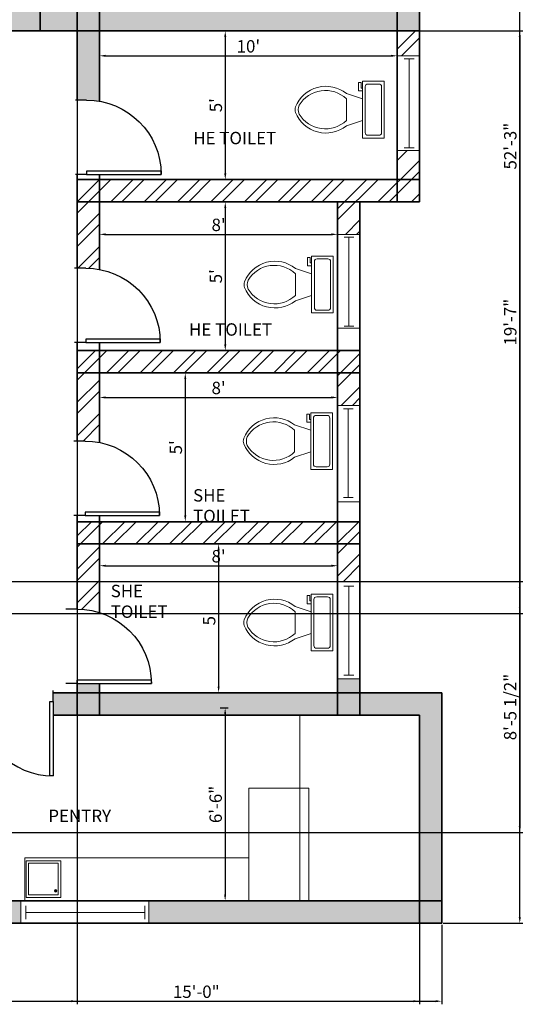
# Model space of a CAD drawing. Units: millimetres. Extents: x 2436 to 3005, y 774 to 1472.
# Tile 2 of 3: x 2799 to 3005, y 774 to 1172. Entities that reach past the tile are written whole.
import ezdxf

# ---------------------------------------------------------------- set-up
doc = ezdxf.new("R2010")
doc.units = ezdxf.units.MM
for name, color, linetype, lineweight in [('A-ANNO-DIMS', 2, 'Continuous', 18), ('A-AREA-IDEN', 10, 'Continuous', 25), ('A-FLOR-CASE', 140, 'Continuous', 18), ('A-FLOR-FIXT', 140, 'Continuous', 18), ('A-WALL-PATT', 3, 'Continuous', 13), ('doors', 30, 'Continuous', 25), ('walls', 80, 'Continuous', 35), ('window', 190, 'Continuous', 20)]:
    doc.layers.add(name, color=color, linetype=linetype, lineweight=lineweight)
doc.styles.get("Standard").update_dxf_attribs({"font": 'arial.ttf'})
doc.dimstyles.new('ISO-25', dxfattribs={"dimtxt": 5, "dimasz": 2.5, "dimexe": 1.25, "dimexo": 0.625, "dimtad": 1, "dimdec": 0, "dimlunit": 3, "dimtxsty": 'Standard', "dimcen": 2.5, "dimadec": 0, "dimazin": 0, "dimtfac": 1, "dimtdec": 0, "dimtmove": 0, "dimatfit": 3, "dimfxl": 1, "dimarcsym": 0})

# ---------------------------------------------------------------- blocks, each defined once
blk = doc.blocks.new('*U2')
for p, q in [((0, 0), (0, -6)), ((40, 0), (40, -6))]:
    blk.add_line(p, q)
blk.add_lwpolyline([(0, 0), (0, 40), (1.75, 40), (1.75, 0)], close=True)
blk.add_arc((0, 0), 40, 0, 90)
blk = doc.blocks.new('*U4')
for p, q in [((0, 4), (0, 0)), ((36, 4), (36, 0)), ((0, 2), (36, 2))]:
    blk.add_line(p, q)
blk = doc.blocks.new('*U5')
for p, q in [((0, 4), (0, 0)), ((36, 4), (36, 0)), ((0, 2), (36, 2))]:
    blk.add_line(p, q)
blk = doc.blocks.new('Toilet - top')
for p, q in [((9.5, -6), (9.5, -2)), ((-10, -8.5), (-8, -8.5)), ((-10, -9.5), (-10, -8.5)), ((-7, -9.5), (-10, -9.5)), ((-8, -8.5), (-8, -8)), ((-7, -8), (-7, -9.5)), ((-4, -8), (-6, -14)), ((4, -8), (6, -14)), ((4, -14), (-4, -14))]:
    blk.add_line(p, q)
blk.add_lwpolyline([(10.5, -8), (10.5, 0), (-10.5, 0), (-10.5, -8)], close=True)
for points in [[(-9.5, -2), (-9.5, -6)], [(8.5, -1), (-8.5, -1)], [(-8.5, -7), (8.5, -7)]]:
    blk.add_lwpolyline(points)
for centre, radius, start, end in [((-8.62, -1.88), 0.884, 81.8699, 188.1301), ((8.62, -1.88), 0.884, 351.8699, 98.1301), ((-8.62, -6.12), 0.884, 171.8699, 278.1301), ((8.62, -6.12), 0.884, 261.8699, 8.1301), ((3.52, -21.58), 12.17, 141.4691, 247.9714), ((4.2, -21.82), 11.33, 136.3677, 238.9468), ((-3.52, -21.58), 12.17, 292.0284, 38.5307), ((-4.2, -21.82), 11.33, 301.053, 43.6321), ((0, -27.88), 4, 245.7318, 294.2682), ((0, -29), 4, 254.8605, 285.1395)]:
    blk.add_arc(centre, radius, start, end)
blk = doc.blocks.new('*D25')
at = {"layer": 'A-ANNO-DIMS', "color": 0, "lineweight": -2, "transparency": 16777216}
for p, q in [((2879.98, 893.97), (2883.19, 893.97)), ((2881.94, 891.47), (2881.94, 818.62)), ((2879.98, 816.12), (2883.19, 816.12))]:
    blk.add_line(p, q, dxfattribs=at)
at = {"layer": 'A-ANNO-DIMS', "color": 0, "transparency": 16777216}
for points in [[(2881.52, 891.47), (2882.35, 891.47), (2881.94, 893.97)], [(2881.52, 818.62), (2882.35, 818.62), (2881.94, 816.12)]]:
    blk.add_solid(points, dxfattribs=at)
at = {"layer": 'Defpoints', "color": 0, "transparency": 16777216}
for p in [(2879.35, 893.97), (2879.35, 816.12), (2881.94, 816.12)]:
    blk.add_point(p, dxfattribs=at)
at = {"layer": 'A-ANNO-DIMS', "color": 0, "transparency": 16777216, "insert": (2878.76, 855.05), "char_height": 5, "attachment_point": 5, "rotation": 90}
blk.add_mtext('6\'-6"', dxfattribs=at)
blk = doc.blocks.new('*D26')
at = {"layer": 'A-ANNO-DIMS', "color": 0, "lineweight": -2, "transparency": 16777216}
for p, q in [((2879.3, 957.62), (2879.3, 902.62)), ((2879.92, 960.12), (2880.55, 960.12)), ((2879.92, 900.12), (2880.55, 900.12))]:
    blk.add_line(p, q, dxfattribs=at)
at = {"layer": 'A-ANNO-DIMS', "color": 0, "transparency": 16777216}
for points in [[(2878.88, 957.62), (2879.72, 957.62), (2879.3, 960.12)], [(2878.88, 902.62), (2879.72, 902.62), (2879.3, 900.12)]]:
    blk.add_solid(points, dxfattribs=at)
at = {"layer": 'Defpoints', "color": 0, "transparency": 16777216}
for p in [(2879.3, 960.12), (2879.3, 900.12), (2879.3, 900.12)]:
    blk.add_point(p, dxfattribs=at)
at = {"layer": 'A-ANNO-DIMS', "color": 0, "transparency": 16777216, "insert": (2876.13, 930.12), "char_height": 5, "attachment_point": 5, "rotation": 90}
blk.add_mtext("5'", dxfattribs=at)
blk = doc.blocks.new('*D27')
at = {"layer": 'A-ANNO-DIMS', "color": 0, "lineweight": -2, "transparency": 16777216}
for p, q in [((2831.3, 1019.85), (2831.3, 1020.48)), ((2833.8, 1019.23), (2924.8, 1019.23)), ((2927.3, 1019.85), (2927.3, 1020.48))]:
    blk.add_line(p, q, dxfattribs=at)
at = {"layer": 'A-ANNO-DIMS', "color": 0, "transparency": 16777216}
for points in [[(2833.8, 1019.65), (2833.8, 1018.81), (2831.3, 1019.23)], [(2924.8, 1019.65), (2924.8, 1018.81), (2927.3, 1019.23)]]:
    blk.add_solid(points, dxfattribs=at)
at = {"layer": 'Defpoints', "color": 0, "transparency": 16777216}
for p in [(2831.3, 1019.23), (2927.3, 1019.23), (2927.3, 1019.23)]:
    blk.add_point(p, dxfattribs=at)
at = {"layer": 'A-ANNO-DIMS', "color": 0, "transparency": 16777216, "insert": (2879.3, 1022.41), "char_height": 5, "attachment_point": 5}
blk.add_mtext("8'", dxfattribs=at)
blk = doc.blocks.new('*D28')
at = {"layer": 'A-ANNO-DIMS', "color": 0, "lineweight": -2, "transparency": 16777216}
for p, q in [((2881.99, 1164.62), (2881.99, 1109.62)), ((2882.61, 1167.12), (2883.24, 1167.12)), ((2882.61, 1107.12), (2883.24, 1107.12))]:
    blk.add_line(p, q, dxfattribs=at)
at = {"layer": 'A-ANNO-DIMS', "color": 0, "transparency": 16777216}
for points in [[(2881.57, 1164.62), (2882.4, 1164.62), (2881.99, 1167.12)], [(2881.57, 1109.62), (2882.4, 1109.62), (2881.99, 1107.12)]]:
    blk.add_solid(points, dxfattribs=at)
at = {"layer": 'Defpoints', "color": 0, "transparency": 16777216}
for p in [(2881.99, 1167.12), (2881.99, 1107.12), (2881.99, 1107.12)]:
    blk.add_point(p, dxfattribs=at)
at = {"layer": 'A-ANNO-DIMS', "color": 0, "transparency": 16777216, "insert": (2878.82, 1137.12), "char_height": 5, "attachment_point": 5, "rotation": 90}
blk.add_mtext("5'", dxfattribs=at)
blk = doc.blocks.new('*D29')
at = {"layer": 'A-ANNO-DIMS', "color": 0, "lineweight": -2, "transparency": 16777216}
for p, q in [((2882.61, 1098.12), (2883.24, 1098.12)), ((2881.99, 1095.62), (2881.99, 1040.62)), ((2882.61, 1038.12), (2883.24, 1038.12))]:
    blk.add_line(p, q, dxfattribs=at)
at = {"layer": 'A-ANNO-DIMS', "color": 0, "transparency": 16777216}
for points in [[(2881.57, 1095.62), (2882.4, 1095.62), (2881.99, 1098.12)], [(2881.57, 1040.62), (2882.4, 1040.62), (2881.99, 1038.12)]]:
    blk.add_solid(points, dxfattribs=at)
at = {"layer": 'Defpoints', "color": 0, "transparency": 16777216}
for p in [(2881.99, 1098.12), (2881.99, 1038.12), (2881.99, 1038.12)]:
    blk.add_point(p, dxfattribs=at)
at = {"layer": 'A-ANNO-DIMS', "color": 0, "transparency": 16777216, "insert": (2878.82, 1068.12), "char_height": 5, "attachment_point": 5, "rotation": 90}
blk.add_mtext("5'", dxfattribs=at)
blk = doc.blocks.new('*D30')
at = {"layer": 'A-ANNO-DIMS', "color": 0, "lineweight": -2, "transparency": 16777216}
for p, q in [((2866.48, 1029.12), (2867.11, 1029.12)), ((2865.86, 1026.62), (2865.86, 971.62)), ((2866.48, 969.12), (2867.11, 969.12))]:
    blk.add_line(p, q, dxfattribs=at)
at = {"layer": 'A-ANNO-DIMS', "color": 0, "transparency": 16777216}
for points in [[(2865.44, 1026.62), (2866.28, 1026.62), (2865.86, 1029.12)], [(2865.44, 971.62), (2866.28, 971.62), (2865.86, 969.12)]]:
    blk.add_solid(points, dxfattribs=at)
at = {"layer": 'Defpoints', "color": 0, "transparency": 16777216}
for p in [(2865.86, 1029.12), (2865.86, 969.12), (2865.86, 969.12)]:
    blk.add_point(p, dxfattribs=at)
at = {"layer": 'A-ANNO-DIMS', "color": 0, "transparency": 16777216, "insert": (2862.69, 999.12), "char_height": 5, "attachment_point": 5, "rotation": 90}
blk.add_mtext("5'", dxfattribs=at)
blk = doc.blocks.new('*D31')
at = {"layer": 'A-ANNO-DIMS', "color": 0, "lineweight": -2, "transparency": 16777216}
for p, q in [((2831.3, 951.41), (2831.3, 950.1)), ((2833.8, 951.35), (2924.8, 951.35)), ((2927.3, 951.98), (2927.3, 952.6))]:
    blk.add_line(p, q, dxfattribs=at)
at = {"layer": 'A-ANNO-DIMS', "color": 0, "transparency": 16777216}
for points in [[(2833.8, 951.77), (2833.8, 950.93), (2831.3, 951.35)], [(2924.8, 951.77), (2924.8, 950.93), (2927.3, 951.35)]]:
    blk.add_solid(points, dxfattribs=at)
at = {"layer": 'Defpoints', "color": 0, "transparency": 16777216}
for p in [(2831.3, 952.04), (2927.3, 951.35), (2927.3, 951.35)]:
    blk.add_point(p, dxfattribs=at)
at = {"layer": 'A-ANNO-DIMS', "color": 0, "transparency": 16777216, "insert": (2879.3, 954.53), "char_height": 5, "attachment_point": 5}
blk.add_mtext("8'", dxfattribs=at)
blk = doc.blocks.new('*D32')
at = {"layer": 'A-ANNO-DIMS', "color": 0, "lineweight": -2, "transparency": 16777216}
for p, q in [((2831.3, 1156.81), (2831.3, 1155.81)), ((2833.8, 1157.06), (2948.8, 1157.06)), ((2951.3, 1156.81), (2951.3, 1155.81))]:
    blk.add_line(p, q, dxfattribs=at)
at = {"layer": 'A-ANNO-DIMS', "color": 0, "transparency": 16777216}
for points in [[(2833.8, 1157.47), (2833.8, 1156.64), (2831.3, 1157.06)], [(2948.8, 1157.47), (2948.8, 1156.64), (2951.3, 1157.06)]]:
    blk.add_solid(points, dxfattribs=at)
at = {"layer": 'Defpoints', "color": 0, "transparency": 16777216}
for p in [(2831.3, 1157.43), (2951.3, 1157.43), (2951.3, 1157.06)]:
    blk.add_point(p, dxfattribs=at)
at = {"layer": 'A-ANNO-DIMS', "color": 0, "transparency": 16777216, "insert": (2891.3, 1160.23), "char_height": 5, "attachment_point": 5}
blk.add_mtext("10'", dxfattribs=at)
blk = doc.blocks.new('*D33')
at = {"layer": 'A-ANNO-DIMS', "color": 0, "lineweight": -2, "transparency": 16777216}
for p, q in [((2831.3, 1087.23), (2831.3, 1083.77)), ((2833.8, 1085.02), (2924.8, 1085.02)), ((2927.3, 1085.65), (2927.3, 1086.27))]:
    blk.add_line(p, q, dxfattribs=at)
at = {"layer": 'A-ANNO-DIMS', "color": 0, "transparency": 16777216}
for points in [[(2833.8, 1085.44), (2833.8, 1084.61), (2831.3, 1085.02)], [(2924.8, 1085.44), (2924.8, 1084.61), (2927.3, 1085.02)]]:
    blk.add_solid(points, dxfattribs=at)
at = {"layer": 'Defpoints', "color": 0, "transparency": 16777216}
for p in [(2831.3, 1087.86), (2927.3, 1085.02), (2927.3, 1085.02)]:
    blk.add_point(p, dxfattribs=at)
at = {"layer": 'A-ANNO-DIMS', "color": 0, "transparency": 16777216, "insert": (2879.3, 1088.2), "char_height": 5, "attachment_point": 5}
blk.add_mtext("8'", dxfattribs=at)
blk = doc.blocks.new('*D40')
at = {"layer": 'A-ANNO-DIMS', "color": 0, "lineweight": -2, "transparency": 16777216}
for p, q in [((2480.3, 806.5), (2480.3, 774.42)), ((2969.3, 806.5), (2969.3, 774.42)), ((2482.8, 775.67), (2966.8, 775.67))]:
    blk.add_line(p, q, dxfattribs=at)
at = {"layer": 'A-ANNO-DIMS', "color": 0, "transparency": 16777216}
for points in [[(2482.8, 776.09), (2482.8, 775.26), (2480.3, 775.67)], [(2966.8, 776.09), (2966.8, 775.26), (2969.3, 775.67)]]:
    blk.add_solid(points, dxfattribs=at)
at = {"layer": 'Defpoints', "color": 0, "transparency": 16777216}
for p in [(2480.3, 807.12), (2969.3, 807.12), (2969.3, 775.67)]:
    blk.add_point(p, dxfattribs=at)
at = {"layer": 'A-ANNO-DIMS', "color": 0, "transparency": 16777216, "insert": (2724.8, 778.85), "char_height": 5, "attachment_point": 5}
blk.add_mtext('40\'-9"', dxfattribs=at)
blk = doc.blocks.new('*D41')
at = {"layer": 'A-ANNO-DIMS', "color": 0, "lineweight": -2, "transparency": 16777216}
for p, q in [((2960.92, 1434.12), (3002, 1434.12)), ((3000.75, 809.62), (3000.75, 1431.62)), ((2969.92, 807.12), (3002, 807.12))]:
    blk.add_line(p, q, dxfattribs=at)
at = {"layer": 'A-ANNO-DIMS', "color": 0, "transparency": 16777216}
for points in [[(3000.33, 1431.62), (3001.17, 1431.62), (3000.75, 1434.12)], [(3000.33, 809.62), (3001.17, 809.62), (3000.75, 807.12)]]:
    blk.add_solid(points, dxfattribs=at)
at = {"layer": 'Defpoints', "color": 0, "transparency": 16777216}
for p in [(2960.3, 1434.12), (3000.75, 1434.12), (2969.3, 807.12)]:
    blk.add_point(p, dxfattribs=at)
at = {"layer": 'A-ANNO-DIMS', "color": 0, "transparency": 16777216, "insert": (2997.57, 1120.62), "char_height": 5, "attachment_point": 5, "rotation": 90}
blk.add_mtext('52\'-3"', dxfattribs=at)
blk = doc.blocks.new('*D42')
at = {"layer": 'A-ANNO-DIMS', "color": 0, "lineweight": -2, "transparency": 16777216}
for p, q in [((2780.3, 931.5), (2780.3, 774.42)), ((2960.3, 890.5), (2960.3, 774.42)), ((2782.8, 775.67), (2957.8, 775.67))]:
    blk.add_line(p, q, dxfattribs=at)
at = {"layer": 'A-ANNO-DIMS', "color": 0, "transparency": 16777216}
for points in [[(2782.8, 776.09), (2782.8, 775.26), (2780.3, 775.67)], [(2957.8, 776.09), (2957.8, 775.26), (2960.3, 775.67)]]:
    blk.add_solid(points, dxfattribs=at)
at = {"layer": 'Defpoints', "color": 0, "transparency": 16777216}
for p in [(2780.3, 932.12), (2960.3, 891.12), (2960.3, 775.67)]:
    blk.add_point(p, dxfattribs=at)
at = {"layer": 'A-ANNO-DIMS', "color": 0, "transparency": 16777216, "insert": (2870.3, 778.85), "char_height": 5, "attachment_point": 5}
blk.add_mtext('15\'-0"', dxfattribs=at)
blk = doc.blocks.new('*D43')
at = {"layer": 'A-ANNO-DIMS', "color": 0, "lineweight": -2, "transparency": 16777216}
for p, q in [((2822.3, 1175.5), (2822.3, 774.42)), ((2618.3, 1160.31), (2618.3, 774.42)), ((2620.8, 775.67), (2819.8, 775.67))]:
    blk.add_line(p, q, dxfattribs=at)
at = {"layer": 'A-ANNO-DIMS', "color": 0, "transparency": 16777216}
for points in [[(2620.8, 776.09), (2620.8, 775.26), (2618.3, 775.67)], [(2819.8, 776.09), (2819.8, 775.26), (2822.3, 775.67)]]:
    blk.add_solid(points, dxfattribs=at)
at = {"layer": 'Defpoints', "color": 0, "transparency": 16777216}
for p in [(2822.3, 1176.12), (2618.3, 1160.93), (2822.3, 775.67)]:
    blk.add_point(p, dxfattribs=at)
at = {"layer": 'A-ANNO-DIMS', "color": 0, "transparency": 16777216, "insert": (2720.3, 778.85), "char_height": 5, "attachment_point": 5}
blk.add_mtext('17\'-0"', dxfattribs=at)
blk = doc.blocks.new('*D44')
at = {"layer": 'A-ANNO-DIMS', "color": 0, "lineweight": -2, "transparency": 16777216}
for p, q in [((2798.92, 1167.12), (3002, 1167.12)), ((3000.75, 1164.62), (3000.75, 934.62)), ((2780.92, 932.12), (3002, 932.12))]:
    blk.add_line(p, q, dxfattribs=at)
at = {"layer": 'A-ANNO-DIMS', "color": 0, "transparency": 16777216}
for points in [[(3000.33, 1164.62), (3001.17, 1164.62), (3000.75, 1167.12)], [(3000.33, 934.62), (3001.17, 934.62), (3000.75, 932.12)]]:
    blk.add_solid(points, dxfattribs=at)
at = {"layer": 'Defpoints', "color": 0, "transparency": 16777216}
for p in [(2798.3, 1167.12), (2780.3, 932.12), (3000.75, 932.12)]:
    blk.add_point(p, dxfattribs=at)
at = {"layer": 'A-ANNO-DIMS', "color": 0, "transparency": 16777216, "insert": (2997.57, 1049.62), "char_height": 5, "attachment_point": 5, "rotation": 90}
blk.add_mtext('19\'-7"', dxfattribs=at)
blk = doc.blocks.new('*D54')
at = {"layer": 'A-ANNO-DIMS', "color": 0, "lineweight": -2, "transparency": 16777216}
for p, q in [((2543.78, 945.02), (3002, 945.02)), ((3000.75, 942.52), (3000.75, 846.17)), ((2543.78, 843.67), (3002, 843.67))]:
    blk.add_line(p, q, dxfattribs=at)
at = {"layer": 'A-ANNO-DIMS', "color": 0, "transparency": 16777216}
for points in [[(3000.33, 942.52), (3001.17, 942.52), (3000.75, 945.02)], [(3000.33, 846.17), (3001.17, 846.17), (3000.75, 843.67)]]:
    blk.add_solid(points, dxfattribs=at)
at = {"layer": 'Defpoints', "color": 0, "transparency": 16777216}
for p in [(2543.16, 945.02), (2543.16, 843.67), (3000.75, 843.67)]:
    blk.add_point(p, dxfattribs=at)
at = {"layer": 'A-ANNO-DIMS', "color": 0, "transparency": 16777216, "insert": (2997.54, 894.35), "char_height": 5, "attachment_point": 5, "rotation": 90}
blk.add_mtext('8\'-5 1/2"', dxfattribs=at)

msp = doc.modelspace()

# ---------------------------------------------------------------- hatches: boundary and pattern name
at = {"layer": 'A-WALL-PATT'}
h = msp.add_hatch(color=256, dxfattribs=at)
h.dxf.hatch_style = 1
h.paths.add_polyline_path([(2822.3, 1374.12), (2489.3, 1374.12), (2489.3, 1365.12), (2822.3, 1365.12)])
h.paths.add_polyline_path([(2831.3, 1374.12), (2822.3, 1374.12), (2822.3, 1365.12), (2831.3, 1365.12)])
h.paths.add_polyline_path([(2831.3, 1365.12), (2822.3, 1365.12), (2822.3, 1353.75), (2824.37, 1353.75, -0.041466), (2831.3, 1353.17)])
h.paths.add_polyline_path([(2960.3, 1425.12), (2951.3, 1425.12), (2951.3, 1305.12), (2960.3, 1305.12)])
h.paths.add_polyline_path([(2960.3, 1434.12), (2951.3, 1434.12), (2951.3, 1425.12), (2960.3, 1425.12)])
h.paths.add_polyline_path([(2951.3, 1434.12), (2831.3, 1434.12), (2831.3, 1425.12), (2951.3, 1425.12)])
h.paths.add_polyline_path([(2831.3, 1434.12), (2822.3, 1434.12), (2822.3, 1425.12), (2831.3, 1425.12)])
h.paths.add_polyline_path([(2489.3, 1374.12), (2480.3, 1374.12), (2480.3, 1365.12), (2489.3, 1365.12)])
h.paths.add_polyline_path([(2489.3, 1365.12), (2480.3, 1365.12), (2480.3, 1354.49), (2489.3, 1354.89)])
h.paths.add_polyline_path([(2489.3, 1313.48, -0.04329), (2482.1, 1312.53), (2480.3, 1312.44), (2480.3, 1176.12), (2489.3, 1176.12)])
h.paths.add_polyline_path([(2489.3, 1176.12), (2480.3, 1176.12), (2480.3, 1167.12), (2489.3, 1167.12)])
h.paths.add_polyline_path([(2609.3, 1176.12), (2489.3, 1176.12), (2489.3, 1167.12), (2609.3, 1167.12)])
h.paths.add_polyline_path([(2625.3, 1176.12), (2618.3, 1176.12), (2618.3, 1167.12), (2625.3, 1167.12)])
h.paths.add_polyline_path([(2618.3, 1176.12), (2616.3, 1176.12), (2616.3, 1167.12), (2618.3, 1167.12)])
h.paths.add_polyline_path([(2616.3, 1176.12), (2609.3, 1176.12), (2609.3, 1167.12), (2616.3, 1167.12)])
h.paths.add_polyline_path([(2618.3, 1167.12), (2609.3, 1167.12), (2609.3, 1160.63, -0.029892), (2614.31, 1160.93), (2618.3, 1160.93)])
h.paths.add_polyline_path([(2625.3, 1305.12), (2616.3, 1305.12), (2616.3, 1176.12), (2618.3, 1176.12), (2625.3, 1176.12)])
h.paths.add_polyline_path([(2798.3, 1176.12), (2625.3, 1176.12), (2625.3, 1167.12), (2798.3, 1167.12)])
h.paths.add_polyline_path([(2807.3, 1176.12), (2798.3, 1176.12), (2798.3, 1167.12), (2807.3, 1167.12)])
h.paths.add_polyline_path([(2831.3, 1176.12), (2822.3, 1176.12), (2822.3, 1167.12), (2831.3, 1167.12)])
h.paths.add_polyline_path([(2822.3, 1176.12), (2807.3, 1176.12), (2807.3, 1167.12), (2822.3, 1167.12)])
h.paths.add_polyline_path([(2951.3, 1176.12), (2831.3, 1176.12), (2831.3, 1167.12), (2951.3, 1167.12)])
h.paths.add_polyline_path([(2960.3, 1176.12), (2951.3, 1176.12), (2951.3, 1167.12), (2960.3, 1167.12)])
h.paths.add_polyline_path([(2960.3, 1296.12), (2951.3, 1296.12), (2951.3, 1176.12), (2960.3, 1176.12)])
h.paths.add_polyline_path([(2960.3, 1305.12), (2951.3, 1305.12), (2951.3, 1296.12), (2960.3, 1296.12)])
h.paths.add_polyline_path([(2951.3, 1305.12), (2831.3, 1305.12), (2831.3, 1296.12), (2951.3, 1296.12)])
h.paths.add_polyline_path([(2822.3, 1305.12), (2807.3, 1305.12), (2807.3, 1296.12), (2822.3, 1296.12)])
h.paths.add_polyline_path([(2831.3, 1305.12), (2822.3, 1305.12), (2822.3, 1296.12), (2831.3, 1296.12)])
h.paths.add_polyline_path([(2831.3, 1311.75), (2824.37, 1311.75), (2822.3, 1311.75), (2822.3, 1305.12), (2831.3, 1305.12)])
h.paths.add_polyline_path([(2807.3, 1305.12), (2798.3, 1305.12), (2798.3, 1296.12), (2807.3, 1296.12)])
h.paths.add_polyline_path([(2807.3, 1236.01), (2798.3, 1236.01), (2798.3, 1221.93), (2801.81, 1221.93, -0.032777), (2807.3, 1221.57)])
h.paths.add_polyline_path([(2831.3, 1167.12), (2822.3, 1167.12), (2822.3, 1139.2), (2826.09, 1139.2, -0.043681), (2831.3, 1138.75)])
h.paths.add_polyline_path([(2807.3, 1179.93), (2801.81, 1179.93), (2798.3, 1179.93), (2798.3, 1176.12), (2807.3, 1176.12)])
h.paths.add_polyline_path([(2927.3, 900.12), (2831.3, 900.12), (2831.3, 891.12), (2927.3, 891.12)])
h.paths.add_polyline_path([(2936.3, 900.12), (2927.3, 900.12), (2927.3, 891.12), (2936.3, 891.12)])
h.paths.add_polyline_path([(2936.3, 905.69), (2927.3, 905.69), (2927.3, 900.12), (2936.3, 900.12)])
h.paths.add_polyline_path([(2831.3, 900.12), (2822.3, 900.12), (2822.3, 891.12), (2831.3, 891.12)])
h.paths.add_polyline_path([(2831.3, 903.84), (2822.3, 903.84), (2822.3, 900.12), (2831.3, 900.12)])
h.paths.add_polyline_path([(2822.3, 900.12), (2812.6, 900.12), (2812.6, 896.54), (2812.6, 891.12), (2822.3, 891.12)])
h.paths.add_polyline_path([(2969.3, 900.12), (2958.95, 900.12), (2936.3, 900.12), (2936.3, 891.12), (2960.3, 891.12), (2960.3, 826.87), (2960.3, 816.12), (2969.3, 816.12), (2969.3, 826.87), (2969.3, 891.12)])
h = msp.add_hatch(color=256, dxfattribs=at)
h.dxf.hatch_style = 1
h.paths.add_polyline_path([(2780.3, 891.12), (2771.3, 891.12), (2771.3, 816.12), (2780.3, 816.12)])
h.paths.add_polyline_path([(2780.3, 900.12), (2771.3, 900.12), (2771.3, 891.12), (2780.3, 891.12)])
h.paths.add_polyline_path([(2780.3, 923.12), (2771.3, 923.12), (2771.3, 900.12), (2780.3, 900.12)])
h.paths.add_polyline_path([(2780.3, 932.12), (2771.3, 932.12), (2771.3, 923.12), (2780.3, 923.12)])
h.paths.add_polyline_path([(2771.3, 932.12), (2687.55, 932.12), (2687.55, 930.04), (2687.55, 923.12), (2771.3, 923.12)])
h.paths.add_polyline_path([(2651.3, 923.12), (2642.3, 923.12), (2642.3, 816.12), (2651.3, 816.12)])
h.paths.add_polyline_path([(2651.3, 816.12), (2642.3, 816.12), (2642.3, 807.12), (2651.3, 807.12)])
h.paths.add_polyline_path([(2771.3, 816.12), (2651.3, 816.12), (2651.3, 807.12), (2771.3, 807.12)])
h.paths.add_polyline_path([(2780.3, 816.12), (2771.3, 816.12), (2771.3, 807.12), (2780.3, 807.12)])
h.paths.add_polyline_path([(2799.5, 816.12), (2780.3, 816.12), (2780.3, 807.12), (2799.5, 807.12)])
h.paths.add_polyline_path([(2960.3, 816.12), (2851.13, 816.12), (2851.13, 807.12), (2960.3, 807.12)])
h.paths.add_polyline_path([(2969.3, 816.12), (2960.3, 816.12), (2960.3, 807.12), (2969.3, 807.12)])
h.paths.add_polyline_path([(2642.3, 816.12), (2489.3, 816.12), (2489.3, 807.12), (2642.3, 807.12)])
h.paths.add_polyline_path([(2489.3, 816.12), (2480.3, 816.12), (2480.3, 807.12), (2489.3, 807.12)])
h.paths.add_polyline_path([(2489.3, 969.12), (2480.3, 969.12), (2480.3, 816.12), (2489.3, 816.12)])
h.paths.add_polyline_path([(2609.3, 978.12), (2489.3, 978.12), (2489.3, 969.12), (2609.3, 969.12)])
h.paths.add_polyline_path([(2489.3, 978.12), (2480.3, 978.12), (2480.3, 969.12), (2489.3, 969.12)])
h.paths.add_polyline_path([(2618.3, 978.12), (2609.3, 978.12), (2609.3, 969.12), (2618.3, 969.12)])
h.paths.add_polyline_path([(2642.3, 978.12), (2618.3, 978.12), (2618.3, 969.12), (2642.3, 969.12)])
h.paths.add_polyline_path([(2651.3, 978.12), (2642.3, 978.12), (2642.3, 969.12), (2651.3, 969.12)])
h.paths.add_polyline_path([(2651.3, 969.12), (2642.3, 969.12), (2642.3, 964.63), (2651.3, 964.63)])
h.paths.add_polyline_path([(2651.3, 932.12), (2642.3, 932.12), (2642.3, 923.12), (2651.3, 923.12)])
h.paths.add_polyline_path([(2657.55, 930.04), (2657.55, 932.12), (2651.3, 932.12), (2651.3, 923.12), (2658.36, 923.12, -0.058212)])
h.paths.add_polyline_path([(2651.3, 938.64, -0.080735), (2642.3, 935.23), (2642.3, 932.12), (2651.3, 932.12)])
h.paths.add_polyline_path([(2489.3, 1038.12), (2480.3, 1038.12), (2480.3, 978.12), (2489.3, 978.12)])
h.paths.add_polyline_path([(2618.3, 987.5), (2609.3, 987.5), (2609.3, 978.12), (2618.3, 978.12)])
h.paths.add_polyline_path([(2618.3, 1038.12), (2609.3, 1038.12), (2609.3, 1026.42), (2618.3, 1026.42)])
h.paths.add_polyline_path([(2489.3, 1047.12), (2480.3, 1047.12), (2480.3, 1038.12), (2489.3, 1038.12)])
h.paths.add_polyline_path([(2618.3, 1047.12), (2609.3, 1047.12), (2609.3, 1038.12), (2618.3, 1038.12)])
h.paths.add_polyline_path([(2489.3, 1167.12), (2480.3, 1167.12), (2480.3, 1047.12), (2489.3, 1047.12)])
h.paths.add_polyline_path([(2618.3, 1118.93), (2614.31, 1118.93), (2609.3, 1118.93), (2609.3, 1108.92), (2618.3, 1108.92)])
h.paths.add_polyline_path([(2618.3, 1056.71), (2609.3, 1056.71), (2609.3, 1047.12), (2618.3, 1047.12)])
edge = h.paths.add_edge_path()
edge.add_arc((2601.4, 1049.98), 30, 185.4674, 203.2834)
edge.add_line((2573.84, 1038.12), (2489.3, 1038.12))
edge.add_line((2489.3, 1038.12), (2489.3, 1047.12))
edge.add_line((2489.3, 1047.12), (2571.54, 1047.12))
h.paths.add_polyline_path([(2601.4, 1047.12), (2601.4, 1038.12), (2609.3, 1038.12), (2609.3, 1047.12)])
h = msp.add_hatch(dxfattribs=at)
h.set_pattern_fill('ANSI32', color=256)
h.paths.add_polyline_path([(2951.3, 1107.12), (2831.3, 1107.12), (2831.3, 1098.12), (2951.3, 1098.12)])
h.paths.add_polyline_path([(2831.3, 1107.12), (2822.3, 1107.12), (2822.3, 1098.12), (2831.3, 1098.12)])
h.paths.add_polyline_path([(2831.3, 1098.12), (2822.3, 1098.12), (2822.3, 1071.38), (2825.75, 1071.38, -0.046499), (2831.3, 1070.86)])
h.paths.add_polyline_path([(2936.3, 1098.12), (2927.3, 1098.12), (2927.3, 1085.02), (2936.3, 1085.02)])
h.paths.add_polyline_path([(2960.3, 1107.12), (2951.3, 1107.12), (2951.3, 1098.12), (2960.3, 1098.12)])
h.paths.add_polyline_path([(2960.3, 1118.92), (2951.3, 1118.92), (2951.3, 1107.12), (2960.3, 1107.12)])
h.paths.add_polyline_path([(2960.3, 1167.12), (2951.3, 1167.12), (2951.3, 1157.06), (2960.3, 1157.06)])
h.paths.add_polyline_path([(2927.3, 1037.38), (2927.3, 1038.12), (2831.3, 1038.12), (2831.3, 1037.38), (2831.3, 1029.12), (2927.3, 1029.12)])
h.paths.add_polyline_path([(2936.3, 1037.38), (2936.3, 1038.12), (2927.3, 1038.12), (2927.3, 1037.38), (2927.3, 1029.12), (2936.3, 1029.12)])
h.paths.add_polyline_path([(2831.3, 1029.12), (2822.3, 1029.12), (2822.3, 1001.65), (2825.44, 1001.65, -0.049211), (2831.3, 1001.07)])
h.paths.add_polyline_path([(2831.3, 1037.38), (2831.3, 1038.12), (2822.3, 1038.12), (2822.3, 1029.12), (2831.3, 1029.12)])
h.paths.add_polyline_path([(2927.3, 969.12), (2831.3, 969.12), (2831.3, 960.12), (2927.3, 960.12)])
h.paths.add_polyline_path([(2831.3, 969.12), (2822.3, 969.12), (2822.3, 960.12), (2831.3, 960.12)])
h.paths.add_polyline_path([(2831.3, 960.12), (2822.3, 960.12), (2822.3, 933.84, -0.076367), (2831.3, 932.43)])
h.paths.add_polyline_path([(2936.3, 969.12), (2927.3, 969.12), (2927.3, 960.12), (2936.3, 960.12)])
h.paths.add_polyline_path([(2936.3, 960.12), (2927.3, 960.12), (2927.3, 945.01), (2936.3, 945.01), (2936.3, 949.23)])
h.paths.add_polyline_path([(2936.3, 1029.12), (2927.3, 1029.12), (2927.3, 1015.96), (2936.3, 1015.96)])

# ---------------------------------------------------------------- linework, layer by layer
at = {"layer": 'A-FLOR-CASE'}
for p, q in [((2912.09, 816.12), (2912.09, 891.12)), ((2891.47, 833.51), (2801.13, 833.51)), ((2801.13, 833.51), (2801.13, 816.12)), ((2801.13, 816.12), (2912.09, 816.12))]:
    msp.add_line(p, q, dxfattribs=at)
msp.add_lwpolyline([(2891.47, 816.12), (2915.69, 816.12), (2915.69, 861.56), (2891.47, 861.56)], close=True, dxfattribs=at)
at = {"layer": 'A-FLOR-FIXT'}
for points in [[(2801.67, 832.31), (2815.64, 832.31), (2815.64, 817.57), (2801.67, 817.57)], [(2802.67, 831.31), (2814.64, 831.31), (2814.64, 818.57), (2802.67, 818.57)]]:
    msp.add_lwpolyline(points, close=True, dxfattribs=at)
for radius in [0.499, 0.13]:
    msp.add_circle((2813.59, 820.2), radius, dxfattribs=at)
at = {"layer": 'walls'}
for p, q in [((2951.3, 1434.12), (2951.3, 1098.12)), ((2960.3, 1434.12), (2960.3, 1098.12)), ((2807.3, 1181.77), (2807.3, 1167.12)), ((2822.3, 1176.12), (2822.3, 1139.2)), ((2831.3, 1176.12), (2831.3, 1138.75)), ((2960.3, 1167.12), (2480.3, 1167.12)), ((2822.3, 1109.2), (2822.3, 1098.12)), ((2831.3, 1109.2), (2831.3, 1098.12)), ((2960.3, 1107.12), (2822.3, 1107.12)), ((2960.3, 1098.12), (2822.3, 1098.12)), ((2822.3, 1098.12), (2822.3, 1071.38)), ((2831.3, 1098.12), (2831.3, 1070.86)), ((2927.3, 1098.12), (2927.3, 1037.38)), ((2960.3, 1098.12), (2936.3, 1098.12)), ((2960.3, 1098.12), (2936.3, 1098.12)), ((2936.3, 1098.12), (2936.3, 1037.38)), ((2822.3, 1041.38), (2822.3, 1001.65)), ((2831.3, 1041.38), (2831.3, 1037.38)), ((2936.3, 1038.12), (2822.3, 1038.12)), ((2831.3, 1037.38), (2831.3, 1001.07)), ((2927.3, 1037.38), (2927.3, 981.58)), ((2936.3, 1037.38), (2936.3, 981.58)), ((2936.3, 1029.12), (2822.3, 1029.12)), ((2927.3, 981.58), (2927.3, 951.35)), ((2936.3, 981.58), (2936.3, 949.23)), ((2822.3, 971.65), (2822.3, 960.12)), ((2831.3, 971.65), (2831.3, 932.43)), ((2936.3, 969.12), (2822.3, 969.12)), ((2936.3, 960.12), (2822.3, 960.12)), ((2822.3, 960.12), (2822.3, 933.84)), ((2927.3, 960.12), (2927.3, 891.12)), ((2936.3, 949.23), (2936.3, 891.12)), ((2822.3, 903.84), (2822.3, 891.12)), ((2831.3, 903.84), (2831.3, 891.12)), ((2936.3, 900.12), (2812.6, 900.12)), ((2936.3, 900.12), (2960.3, 900.12)), ((2969.3, 900.12), (2958.95, 900.12)), ((2969.3, 891.12), (2969.3, 900.12)), ((2936.3, 891.12), (2812.6, 891.12)), ((2936.3, 891.12), (2960.3, 891.12)), ((2960.3, 891.12), (2960.3, 826.87)), ((2969.3, 891.12), (2969.3, 826.87)), ((2960.3, 826.87), (2960.3, 807.12)), ((2969.3, 826.87), (2969.3, 816.12)), ((2969.3, 816.12), (2480.3, 816.12)), ((2969.3, 816.12), (2969.3, 807.12)), ((2969.3, 807.12), (2480.3, 807.12))]:
    msp.add_line(p, q, dxfattribs=at)
at = {"layer": 'window'}
for p, q in [((2951.3, 1157.06), (2960.3, 1157.06)), ((2951.3, 1118.92), (2960.3, 1118.92)), ((2936.3, 1085.02), (2927.3, 1085.02)), ((2927.3, 1047.22), (2936.3, 1047.22)), ((2936.3, 1015.96), (2927.3, 1015.96)), ((2936.3, 977.15), (2927.3, 977.15)), ((2936.3, 945.01), (2927.3, 945.01)), ((2936.3, 905.69), (2927.3, 905.69)), ((2799.5, 816.12), (2799.5, 807.12)), ((2851.13, 816.12), (2851.13, 807.12))]:
    msp.add_line(p, q, dxfattribs=at)

# ---------------------------------------------------------------- block references
at = {"layer": 'A-FLOR-FIXT', "xscale": 1.089104113419681, "yscale": 1.089104113419681, "zscale": 1.089104113419681, "rotation": 270}
for p in [(2946.08, 1135.33), (2925.53, 1064.76), (2925.21, 1001.62), (2925.38, 928.42)]:
    msp.add_blockref('Toilet - top', p, dxfattribs=at)
at = {"layer": 'doors', "yscale": 0.75, "zscale": 0.75}
for p, xscale, rotation in [((2826.09, 1109.2), -0.75, 270), ((2825.75, 1041.38), -0.75, 270), ((2825.44, 971.65), -0.75, 270), ((2822.19, 903.84), -0.75, 270), ((2812.6, 896.54), 0.75, 180)]:
    msp.add_blockref('*U2', p, dxfattribs=dict(at, xscale=xscale, rotation=rotation))
at = {"layer": 'window'}
for name, p, xscale, yscale, zscale, rotation in [('*U5', (2958.11, 1119.95), 0.9968650679331311, 0.9968650679331311, 0.9968650679331311, 90), ('*U5', (2933.87, 1048.05), 0.9968650679331311, 0.9968650679331311, 0.9968650679331311, 90), ('*U5', (2933.6, 978.82), 0.9968650679331311, 0.9968650679331311, 0.9968650679331311, 90), ('*U5', (2933.82, 907.25), 0.9968650679331311, 0.9968650679331311, 0.9968650679331311, 90), ('*U4', (2849.51, 814.17), 1.333333333333333, 1.333333333333333, 1.333333333333333, 180)]:
    msp.add_blockref(name, p, dxfattribs=dict(at, xscale=xscale, yscale=yscale, zscale=zscale, rotation=rotation))

# ---------------------------------------------------------------- texts
at = {"layer": 'A-AREA-IDEN', "char_height": 5, "attachment_point": 1}
for s, width, insert in [('HE TOILET', 47.6796, (2869.07, 1126.38)), ('HE TOILET', 37.3254, (2867.4, 1049.15)), ('SHE TOILET', 35.8326, (2869, 982.24)), ('SHE TOILET', 32.1575, (2835.79, 943.65)), ('PENTRY', 64.4947, (2810.63, 852.94))]:
    msp.add_mtext_dynamic_manual_height_columns(s, width=width, gutter_width=12.5, heights=[0], dxfattribs=dict(at, insert=insert))

# ---------------------------------------------------------------- dimensions: what is measured, and where the dimension line sits
at = {"layer": 'A-ANNO-DIMS'}
for base, p1, p2, override, picture, middle in [((3000.75, 1434.12), (2969.3, 807.12), (2960.3, 1434.12), {"dimdec": 1, "dimlfac": 1, "dimrnd": 0, "dimzin": 1, "dimdsep": 46, "dimlunit": 4, "dimfrac": 2}, '*D41', (2997.57, 1120.62)), ((3000.75, 932.12), (2798.3, 1167.12), (2780.3, 932.12), {"dimdec": 1, "dimlfac": 1, "dimrnd": 0, "dimzin": 1, "dimdsep": 46, "dimlunit": 4, "dimfrac": 2}, '*D44', (2997.57, 1049.62)), ((2881.99, 1107.12), (2881.99, 1167.12), (2881.99, 1107.12), {"dimclrd": 0, "dimclre": 0, "dimclrt": 0}, '*D28', (2878.82, 1137.12)), ((2881.99, 1038.12), (2881.99, 1098.12), (2881.99, 1038.12), {"dimclrd": 0, "dimclre": 0, "dimclrt": 0}, '*D29', (2878.82, 1068.12)), ((2865.86, 969.12), (2865.86, 1029.12), (2865.86, 969.12), {"dimclrd": 0, "dimclre": 0, "dimclrt": 0}, '*D30', (2862.69, 999.12)), ((2879.3, 900.12), (2879.3, 960.12), (2879.3, 900.12), {"dimclrd": 0, "dimclre": 0, "dimclrt": 0}, '*D26', (2876.13, 930.12)), ((3000.7486, 843.6717), (2543.1562, 945.023), (2543.1562, 843.6717), {"dimdec": 1, "dimlfac": 1, "dimrnd": 0, "dimzin": 1, "dimdsep": 46, "dimlunit": 4, "dimfrac": 2}, '*D54', (2997.5383, 894.3473)), ((2881.94, 816.12), (2879.35, 893.97), (2879.35, 816.12), {"dimclrd": 0, "dimclre": 0, "dimclrt": 0}, '*D25', (2878.76, 855.05))]:
    dim = msp.add_linear_dim(base=base, p1=p1, p2=p2, angle=90, dimstyle='ISO-25', override=override, dxfattribs=at)
    dim.commit()
    dim.dimension.update_dxf_attribs({"geometry": picture, "text_midpoint": middle})
for base, p1, p2, override, picture, middle in [((2822.3, 775.67), (2618.3, 1160.93), (2822.3, 1176.12), {"dimdec": 1, "dimlfac": 1, "dimrnd": 0, "dimzin": 1, "dimdsep": 46, "dimlunit": 4, "dimfrac": 2}, '*D43', (2720.3, 778.85)), ((2951.3, 1157.06), (2831.3, 1157.43), (2951.3, 1157.43), {"dimclrd": 0, "dimclre": 0, "dimclrt": 0}, '*D32', (2891.3, 1160.23)), ((2927.3, 1085.02), (2831.3, 1087.86), (2927.3, 1085.02), {"dimclrd": 0, "dimclre": 0, "dimclrt": 0}, '*D33', (2879.3, 1088.2)), ((2927.3, 1019.23), (2831.3, 1019.23), (2927.3, 1019.23), {"dimclrd": 0, "dimclre": 0, "dimclrt": 0}, '*D27', (2879.3, 1022.41)), ((2927.3, 951.35), (2831.3, 952.04), (2927.3, 951.35), {"dimclrd": 0, "dimclre": 0, "dimclrt": 0}, '*D31', (2879.3, 954.53)), ((2960.3, 775.67), (2780.3, 932.12), (2960.3, 891.12), {"dimdec": 1, "dimlfac": 1, "dimrnd": 0, "dimzin": 1, "dimdsep": 46, "dimlunit": 4, "dimfrac": 2}, '*D42', (2870.3, 778.85)), ((2969.3, 775.67), (2480.3, 807.12), (2969.3, 807.12), {"dimdec": 1, "dimlfac": 1, "dimrnd": 0, "dimzin": 1, "dimdsep": 46, "dimlunit": 4, "dimfrac": 2}, '*D40', (2724.8, 778.85))]:
    dim = msp.add_linear_dim(base=base, p1=p1, p2=p2, dimstyle='ISO-25', override=override, dxfattribs=at)
    dim.commit()
    dim.dimension.update_dxf_attribs({"geometry": picture, "text_midpoint": middle})

doc.saveas('drawing.dxf')
